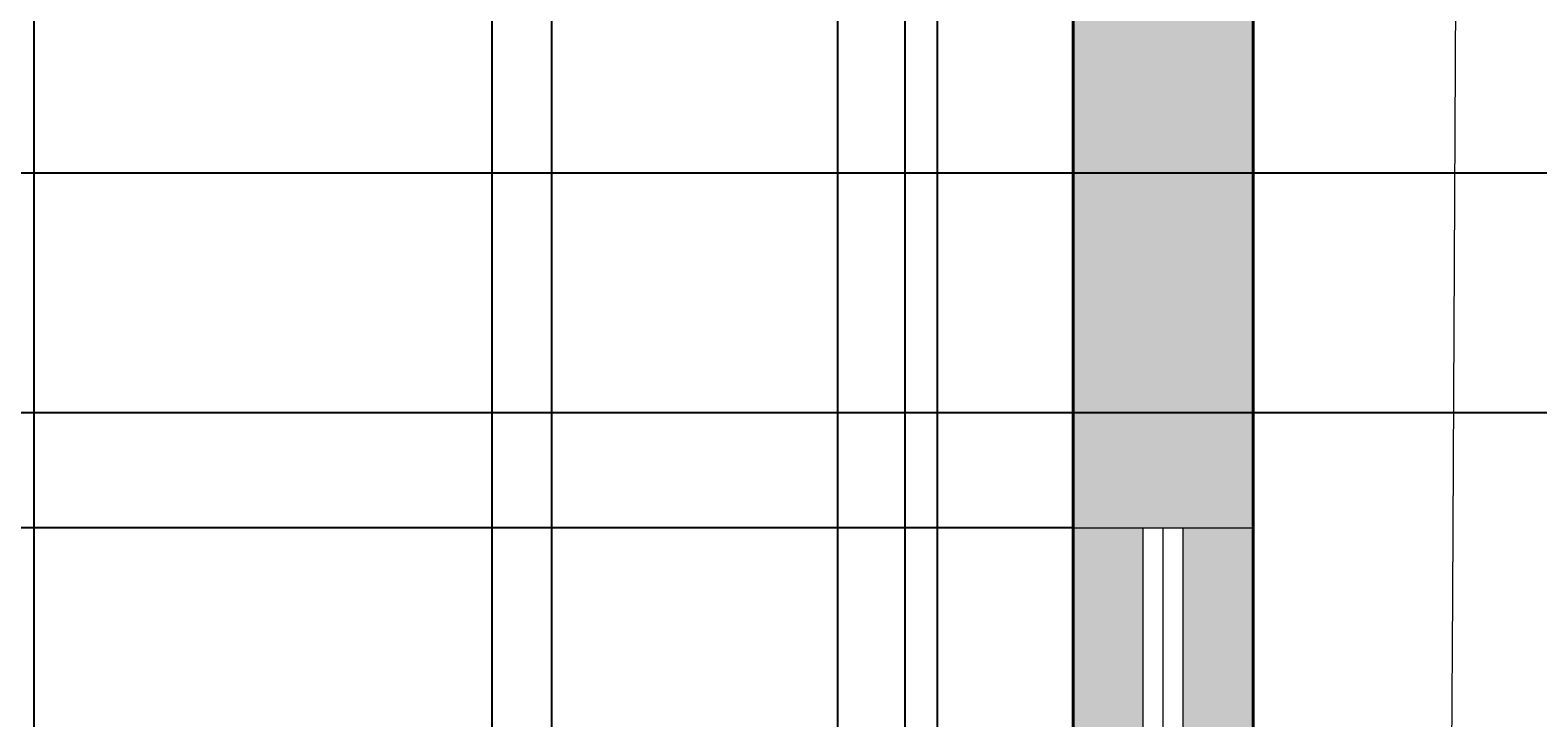
# Model space of a CAD drawing. Units: inches. Extents: x 818 to 1898, y 976 to 2364.
# Tile 30 of 96: x 1207 to 1282, y 1746 to 1780. Entities that reach past the tile are written whole.
import ezdxf

# ---------------------------------------------------------------- set-up
doc = ezdxf.new("R2010")
doc.units = ezdxf.units.IN
doc.header["$LTSCALE"] = 5
doc.header["$MEASUREMENT"] = 0
for name, color, linetype, lineweight in [('A-ANNO-DIMS', 2, 'Continuous', 18), ('A-FURN', 8, 'Continuous', 18), ('A-GLAZ', 4, 'Continuous', 18), ('A-WALL', 7, 'Continuous', 40)]:
    doc.layers.add(name, color=color, linetype=linetype, lineweight=lineweight)
doc.layers.add('A-GLAZ-PATT', color=141, linetype='Continuous', lineweight=9, true_color=0xadddf7)
doc.layers.add('A-WALL-PATT', color=251, linetype='Continuous', lineweight=13, true_color=0x636466)
doc.styles.get("Standard").update_dxf_attribs({"font": 'arial.ttf'})
doc.dimstyles.get("Standard").update_dxf_attribs({"dimtxt": 0.18, "dimasz": 0.18, "dimexe": 0.18, "dimexo": 0.0625, "dimgap": 0.09, "dimtad": 0, "dimtih": 1, "dimtoh": 1, "dimdec": 4, "dimzin": 0, "dimdsep": 46, "dimtxsty": 'Standard', "dimcen": 0.09, "dimadec": 0, "dimazin": 0, "dimtfac": 1, "dimtdec": 4, "dimtofl": 0, "dimtmove": 0, "dimatfit": 3, "dimfxl": 1, "dimtolj": 1, "dimtzin": 0, "dimarcsym": 0})

# ---------------------------------------------------------------- blocks, each defined once
blk = doc.blocks.new('SOFA-3-SEAT')
for p, q in [((39.87, 35.861), (5.697, 36.046)), ((74.051, 35.676), (39.879, 35.861))]:
    blk.add_line(p, q)
blk = doc.blocks.new('*D59')
at = {"layer": 'A-ANNO-DIMS', "color": 0, "lineweight": -2, "ltscale": 5, "transparency": 16777216}
for p, q in [((1251.643, 2300.393), (818.026, 2300.393)), ((818.206, 2300.213), (818.206, 1669.95)), ((818.206, 1039.323), (818.206, 1669.586)), ((896.051, 1039.143), (818.026, 1039.143))]:
    blk.add_line(p, q, dxfattribs=at)
at = {"layer": 'A-ANNO-DIMS', "color": 0, "ltscale": 5, "transparency": 16777216}
for points in [[(818.176, 2300.213), (818.236, 2300.213), (818.206, 2300.393)], [(818.176, 1039.323), (818.236, 1039.323), (818.206, 1039.143)]]:
    blk.add_solid(points, dxfattribs=at)
at = {"layer": 'Defpoints', "color": 0, "ltscale": 5, "transparency": 16777216}
for p in [(818.206, 2300.393), (1251.706, 2300.393), (896.114, 1039.143)]:
    blk.add_point(p, dxfattribs=at)
at = {"layer": 'A-ANNO-DIMS', "color": 0, "ltscale": 5, "transparency": 16777216, "insert": (818.206, 1669.768), "char_height": 0.18, "attachment_point": 5}
blk.add_mtext('\\A1;1261.2', dxfattribs=at)
blk = doc.blocks.new('*D61')
at = {"layer": 'A-ANNO-DIMS', "color": 0, "lineweight": -2, "ltscale": 5, "transparency": 16777216}
for p, q in [((1071.725, 1203.027), (1071.725, 2363.873)), ((1430.725, 1203.027), (1430.725, 2363.873)), ((1071.905, 2363.693), (1250.936, 2363.693)), ((1430.545, 2363.693), (1251.514, 2363.693))]:
    blk.add_line(p, q, dxfattribs=at)
at = {"layer": 'A-ANNO-DIMS', "color": 0, "ltscale": 5, "transparency": 16777216}
for points in [[(1071.905, 2363.723), (1071.905, 2363.663), (1071.725, 2363.693)], [(1430.545, 2363.723), (1430.545, 2363.663), (1430.725, 2363.693)]]:
    blk.add_solid(points, dxfattribs=at)
at = {"layer": 'Defpoints', "color": 0, "ltscale": 5, "transparency": 16777216}
for p in [(1430.725, 2363.693), (1071.725, 1202.964), (1430.725, 1202.964)]:
    blk.add_point(p, dxfattribs=at)
at = {"layer": 'A-ANNO-DIMS', "color": 0, "ltscale": 5, "transparency": 16777216, "insert": (1251.225, 2363.693), "char_height": 0.18, "attachment_point": 5}
blk.add_mtext('\\A1;359', dxfattribs=at)
blk = doc.blocks.new('*D64')
at = {"layer": 'A-ANNO-DIMS', "color": 0, "lineweight": -2, "ltscale": 5, "transparency": 16777216}
for p, q in [((1197.725, 1501.141), (1197.725, 2363.873)), ((1430.725, 1501.141), (1430.725, 2363.873)), ((1197.905, 2363.693), (1313.935, 2363.693)), ((1430.545, 2363.693), (1314.516, 2363.693))]:
    blk.add_line(p, q, dxfattribs=at)
at = {"layer": 'A-ANNO-DIMS', "color": 0, "ltscale": 5, "transparency": 16777216}
for points in [[(1197.905, 2363.723), (1197.905, 2363.663), (1197.725, 2363.693)], [(1430.545, 2363.723), (1430.545, 2363.663), (1430.725, 2363.693)]]:
    blk.add_solid(points, dxfattribs=at)
at = {"layer": 'Defpoints', "color": 0, "ltscale": 5, "transparency": 16777216}
for p in [(1430.725, 2363.693), (1197.725, 1501.078), (1430.725, 1501.078)]:
    blk.add_point(p, dxfattribs=at)
at = {"layer": 'A-ANNO-DIMS', "color": 0, "ltscale": 5, "transparency": 16777216, "insert": (1314.225, 2363.693), "char_height": 0.18, "attachment_point": 5}
blk.add_mtext('\\A1;233', dxfattribs=at)
blk = doc.blocks.new('*D83')
at = {"layer": 'A-ANNO-DIMS', "color": 0, "lineweight": -2, "ltscale": 5, "transparency": 16777216}
for p, q in [((1197.725, 1700.141), (1197.725, 2363.873)), ((1258.725, 1700.141), (1258.725, 2363.873)), ((1197.905, 2363.693), (1228.023, 2363.693)), ((1258.545, 2363.693), (1228.427, 2363.693))]:
    blk.add_line(p, q, dxfattribs=at)
at = {"layer": 'A-ANNO-DIMS', "color": 0, "ltscale": 5, "transparency": 16777216}
for points in [[(1197.905, 2363.723), (1197.905, 2363.663), (1197.725, 2363.693)], [(1258.545, 2363.723), (1258.545, 2363.663), (1258.725, 2363.693)]]:
    blk.add_solid(points, dxfattribs=at)
at = {"layer": 'Defpoints', "color": 0, "ltscale": 5, "transparency": 16777216}
for p in [(1258.725, 2363.693), (1197.725, 1700.078), (1258.725, 1700.078)]:
    blk.add_point(p, dxfattribs=at)
at = {"layer": 'A-ANNO-DIMS', "color": 0, "ltscale": 5, "transparency": 16777216, "insert": (1228.225, 2363.693), "char_height": 0.18, "attachment_point": 5}
blk.add_mtext('\\A1;61', dxfattribs=at)
blk = doc.blocks.new('*D85')
at = {"layer": 'A-ANNO-DIMS', "color": 0, "lineweight": -2, "ltscale": 5, "transparency": 16777216}
for p, q in [((1258.788, 2053.078), (1897.916, 2053.078)), ((1897.736, 2052.898), (1897.736, 1876.76)), ((1897.736, 1700.258), (1897.736, 1876.396)), ((1258.788, 1700.078), (1897.916, 1700.078))]:
    blk.add_line(p, q, dxfattribs=at)
at = {"layer": 'A-ANNO-DIMS', "color": 0, "ltscale": 5, "transparency": 16777216}
for points in [[(1897.706, 2052.898), (1897.766, 2052.898), (1897.736, 2053.078)], [(1897.706, 1700.258), (1897.766, 1700.258), (1897.736, 1700.078)]]:
    blk.add_solid(points, dxfattribs=at)
at = {"layer": 'Defpoints', "color": 0, "ltscale": 5, "transparency": 16777216}
for p in [(1258.725, 2053.078), (1897.736, 2053.078), (1258.725, 1700.078)]:
    blk.add_point(p, dxfattribs=at)
at = {"layer": 'A-ANNO-DIMS', "color": 0, "ltscale": 5, "transparency": 16777216, "insert": (1897.736, 1876.578), "char_height": 0.18, "attachment_point": 5}
blk.add_mtext('\\A1;353', dxfattribs=at)
blk = doc.blocks.new('*D95')
at = {"layer": 'A-ANNO-DIMS', "color": 0, "lineweight": -2, "ltscale": 5, "transparency": 16777216}
for p, q in [((1173.542, 1071.118), (1173.542, 2363.873)), ((1229.647, 1071.118), (1229.647, 2363.873)), ((1173.722, 2363.693), (1201.288, 2363.693)), ((1229.467, 2363.693), (1201.901, 2363.693))]:
    blk.add_line(p, q, dxfattribs=at)
at = {"layer": 'A-ANNO-DIMS', "color": 0, "ltscale": 5, "transparency": 16777216}
for points in [[(1173.722, 2363.723), (1173.722, 2363.663), (1173.542, 2363.693)], [(1229.467, 2363.723), (1229.467, 2363.663), (1229.647, 2363.693)]]:
    blk.add_solid(points, dxfattribs=at)
at = {"layer": 'Defpoints', "color": 0, "ltscale": 5, "transparency": 16777216}
for p in [(1229.647, 2363.693), (1173.542, 1071.055), (1229.647, 1071.055)]:
    blk.add_point(p, dxfattribs=at)
at = {"layer": 'A-ANNO-DIMS', "color": 0, "ltscale": 5, "transparency": 16777216, "insert": (1201.595, 2363.693), "char_height": 0.18, "attachment_point": 5}
blk.add_mtext('\\A1;56.1', dxfattribs=at)
blk = doc.blocks.new('*D96')
at = {"layer": 'A-ANNO-DIMS', "color": 0, "lineweight": -2, "ltscale": 5, "transparency": 16777216}
for p, q in [((1229.647, 1071.118), (1229.647, 2363.873)), ((1284.17, 1071.118), (1284.17, 2363.873)), ((1229.827, 2363.693), (1256.516, 2363.693)), ((1283.99, 2363.693), (1257.301, 2363.693))]:
    blk.add_line(p, q, dxfattribs=at)
at = {"layer": 'A-ANNO-DIMS', "color": 0, "ltscale": 5, "transparency": 16777216}
for points in [[(1229.827, 2363.723), (1229.827, 2363.663), (1229.647, 2363.693)], [(1283.99, 2363.723), (1283.99, 2363.663), (1284.17, 2363.693)]]:
    blk.add_solid(points, dxfattribs=at)
at = {"layer": 'Defpoints', "color": 0, "ltscale": 5, "transparency": 16777216}
for p in [(1284.17, 2363.693), (1229.647, 1071.055), (1284.17, 1071.055)]:
    blk.add_point(p, dxfattribs=at)
at = {"layer": 'A-ANNO-DIMS', "color": 0, "ltscale": 5, "transparency": 16777216, "insert": (1256.909, 2363.693), "char_height": 0.18, "attachment_point": 5}
blk.add_mtext('\\A1;54.52', dxfattribs=at)
blk = doc.blocks.new('*D120')
at = {"layer": 'A-ANNO-DIMS', "color": 0, "lineweight": -2, "ltscale": 5, "transparency": 16777216}
for p, q in [((1766.29, 1797.717), (818.026, 1797.717)), ((818.206, 1797.537), (818.206, 1757.534)), ((818.206, 1717.167), (818.206, 1757.17)), ((1766.29, 1716.987), (818.026, 1716.987))]:
    blk.add_line(p, q, dxfattribs=at)
at = {"layer": 'A-ANNO-DIMS', "color": 0, "ltscale": 5, "transparency": 16777216}
for points in [[(818.176, 1797.537), (818.236, 1797.537), (818.206, 1797.717)], [(818.176, 1717.167), (818.236, 1717.167), (818.206, 1716.987)]]:
    blk.add_solid(points, dxfattribs=at)
at = {"layer": 'Defpoints', "color": 0, "ltscale": 5, "transparency": 16777216}
for p in [(818.206, 1797.717), (1766.352, 1797.717), (1766.352, 1716.987)]:
    blk.add_point(p, dxfattribs=at)
at = {"layer": 'A-ANNO-DIMS', "color": 0, "ltscale": 5, "transparency": 16777216, "insert": (818.206, 1757.352), "char_height": 0.18, "attachment_point": 5}
blk.add_mtext('\\A1;80.73', dxfattribs=at)
blk = doc.blocks.new('*D145')
at = {"layer": 'A-ANNO-DIMS', "color": 0, "lineweight": -2, "ltscale": 5, "transparency": 16777216}
for p, q in [((1197.393, 2122.314), (1197.393, 975.663)), ((1232.609, 2122.314), (1232.609, 975.663)), ((1197.573, 975.843), (1214.608, 975.843)), ((1232.429, 975.843), (1215.394, 975.843))]:
    blk.add_line(p, q, dxfattribs=at)
at = {"layer": 'A-ANNO-DIMS', "color": 0, "ltscale": 5, "transparency": 16777216}
for points in [[(1197.573, 975.873), (1197.573, 975.813), (1197.393, 975.843)], [(1232.429, 975.873), (1232.429, 975.813), (1232.609, 975.843)]]:
    blk.add_solid(points, dxfattribs=at)
at = {"layer": 'Defpoints', "color": 0, "ltscale": 5, "transparency": 16777216}
for p in [(1197.393, 2122.377), (1232.609, 2122.377), (1232.609, 975.843)]:
    blk.add_point(p, dxfattribs=at)
at = {"layer": 'A-ANNO-DIMS', "color": 0, "ltscale": 5, "transparency": 16777216, "insert": (1215.001, 975.843), "char_height": 0.18, "attachment_point": 5}
blk.add_mtext('\\A1;35.22', dxfattribs=at)
blk = doc.blocks.new('*D215')
at = {"layer": 'A-ANNO-DIMS', "color": 0, "lineweight": -2, "ltscale": 5, "transparency": 16777216}
for p, q in [((1590.663, 1876.078), (818.026, 1876.078)), ((818.206, 1875.898), (818.206, 1781.76)), ((818.206, 1687.258), (818.206, 1781.396)), ((1511.663, 1687.078), (818.026, 1687.078))]:
    blk.add_line(p, q, dxfattribs=at)
at = {"layer": 'A-ANNO-DIMS', "color": 0, "ltscale": 5, "transparency": 16777216}
for points in [[(818.176, 1875.898), (818.236, 1875.898), (818.206, 1876.078)], [(818.176, 1687.258), (818.236, 1687.258), (818.206, 1687.078)]]:
    blk.add_solid(points, dxfattribs=at)
at = {"layer": 'Defpoints', "color": 0, "ltscale": 5, "transparency": 16777216}
for p in [(818.206, 1876.078), (1590.725, 1876.078), (1511.725, 1687.078)]:
    blk.add_point(p, dxfattribs=at)
at = {"layer": 'A-ANNO-DIMS', "color": 0, "ltscale": 5, "transparency": 16777216, "insert": (818.206, 1781.578), "char_height": 0.18, "attachment_point": 5}
blk.add_mtext('\\A1;189', dxfattribs=at)
blk = doc.blocks.new('*D220')
at = {"layer": 'A-ANNO-DIMS', "color": 0, "lineweight": -2, "ltscale": 5, "transparency": 16777216}
for p, q in [((1520.663, 1773.078), (818.026, 1773.078)), ((818.206, 1772.898), (818.206, 1767.259)), ((818.206, 1761.258), (818.206, 1766.898)), ((1520.663, 1761.078), (818.026, 1761.078))]:
    blk.add_line(p, q, dxfattribs=at)
at = {"layer": 'A-ANNO-DIMS', "color": 0, "ltscale": 5, "transparency": 16777216}
for points in [[(818.176, 1772.898), (818.236, 1772.898), (818.206, 1773.078)], [(818.176, 1761.258), (818.236, 1761.258), (818.206, 1761.078)]]:
    blk.add_solid(points, dxfattribs=at)
at = {"layer": 'Defpoints', "color": 0, "ltscale": 5, "transparency": 16777216}
for p in [(818.206, 1773.078), (1520.725, 1773.078), (1520.725, 1761.078)]:
    blk.add_point(p, dxfattribs=at)
at = {"layer": 'A-ANNO-DIMS', "color": 0, "ltscale": 5, "transparency": 16777216, "insert": (818.206, 1767.078), "char_height": 0.18, "attachment_point": 5}
blk.add_mtext('\\A1;12', dxfattribs=at)
blk = doc.blocks.new('*D233')
at = {"layer": 'A-ANNO-DIMS', "color": 0, "lineweight": -2, "ltscale": 5, "transparency": 16777216}
for p, q in [((1267.725, 2044.016), (1267.725, 975.663)), ((1303.931, 2008.329), (1303.931, 975.663)), ((1267.905, 975.843), (1285.365, 975.843)), ((1303.751, 975.843), (1286.292, 975.843))]:
    blk.add_line(p, q, dxfattribs=at)
at = {"layer": 'A-ANNO-DIMS', "color": 0, "ltscale": 5, "transparency": 16777216}
for points in [[(1267.905, 975.873), (1267.905, 975.813), (1267.725, 975.843)], [(1303.751, 975.873), (1303.751, 975.813), (1303.931, 975.843)]]:
    blk.add_solid(points, dxfattribs=at)
at = {"layer": 'Defpoints', "color": 0, "ltscale": 5, "transparency": 16777216}
for p in [(1267.725, 2044.078), (1303.931, 2008.392), (1303.931, 975.843)]:
    blk.add_point(p, dxfattribs=at)
at = {"layer": 'A-ANNO-DIMS', "color": 0, "ltscale": 5, "transparency": 16777216, "insert": (1285.828, 975.843), "char_height": 0.18, "attachment_point": 5}
blk.add_mtext('\\A1;36.206', dxfattribs=at)
blk = doc.blocks.new('*D246')
at = {"layer": 'A-ANNO-DIMS', "color": 0, "lineweight": -2, "ltscale": 5, "transparency": 16777216}
for p, q in [((1258.663, 1755.332), (818.026, 1755.332)), ((818.206, 1755.152), (818.206, 1731.514)), ((818.206, 1707.512), (818.206, 1731.15)), ((1258.663, 1707.332), (818.026, 1707.332))]:
    blk.add_line(p, q, dxfattribs=at)
at = {"layer": 'A-ANNO-DIMS', "color": 0, "ltscale": 5, "transparency": 16777216}
for points in [[(818.176, 1755.152), (818.236, 1755.152), (818.206, 1755.332)], [(818.176, 1707.512), (818.236, 1707.512), (818.206, 1707.332)]]:
    blk.add_solid(points, dxfattribs=at)
at = {"layer": 'Defpoints', "color": 0, "ltscale": 5, "transparency": 16777216}
for p in [(818.206, 1755.332), (1258.725, 1755.332), (1258.725, 1707.332)]:
    blk.add_point(p, dxfattribs=at)
at = {"layer": 'A-ANNO-DIMS', "color": 0, "ltscale": 5, "transparency": 16777216, "insert": (818.206, 1731.332), "char_height": 0.18, "attachment_point": 5}
blk.add_mtext('\\A1;48', dxfattribs=at)
blk = doc.blocks.new('*D249')
at = {"layer": 'A-ANNO-DIMS', "color": 0, "lineweight": -2, "ltscale": 5, "transparency": 16777216}
for p, q in [((1258.663, 1814.965), (818.026, 1814.965)), ((818.206, 1814.785), (818.206, 1785.331)), ((818.206, 1755.512), (818.206, 1784.967)), ((1258.663, 1755.332), (818.026, 1755.332))]:
    blk.add_line(p, q, dxfattribs=at)
at = {"layer": 'A-ANNO-DIMS', "color": 0, "ltscale": 5, "transparency": 16777216}
for points in [[(818.176, 1814.785), (818.236, 1814.785), (818.206, 1814.965)], [(818.176, 1755.512), (818.236, 1755.512), (818.206, 1755.332)]]:
    blk.add_solid(points, dxfattribs=at)
at = {"layer": 'Defpoints', "color": 0, "ltscale": 5, "transparency": 16777216}
for p in [(818.206, 1814.965), (1258.725, 1814.965), (1258.725, 1755.332)]:
    blk.add_point(p, dxfattribs=at)
at = {"layer": 'A-ANNO-DIMS', "color": 0, "ltscale": 5, "transparency": 16777216, "insert": (818.206, 1785.149), "char_height": 0.18, "attachment_point": 5}
blk.add_mtext('\\A1;59.63', dxfattribs=at)
blk = doc.blocks.new('*D251')
at = {"layer": 'A-ANNO-DIMS', "color": 0, "lineweight": -2, "ltscale": 5, "transparency": 16777216}
for p, q in [((1250.303, 1878.329), (1250.303, 975.663)), ((1258.725, 1878.329), (1258.725, 975.663)), ((1250.483, 975.843), (1254.121, 975.843)), ((1258.545, 975.843), (1254.907, 975.843))]:
    blk.add_line(p, q, dxfattribs=at)
at = {"layer": 'A-ANNO-DIMS', "color": 0, "ltscale": 5, "transparency": 16777216}
for points in [[(1250.483, 975.873), (1250.483, 975.813), (1250.303, 975.843)], [(1258.545, 975.873), (1258.545, 975.813), (1258.725, 975.843)]]:
    blk.add_solid(points, dxfattribs=at)
at = {"layer": 'Defpoints', "color": 0, "ltscale": 5, "transparency": 16777216}
for p in [(1250.303, 1878.392), (1258.725, 1878.392), (1258.725, 975.843)]:
    blk.add_point(p, dxfattribs=at)
at = {"layer": 'A-ANNO-DIMS', "color": 0, "ltscale": 5, "transparency": 16777216, "insert": (1254.514, 975.843), "char_height": 0.18, "attachment_point": 5}
blk.add_mtext('\\A1;8.422', dxfattribs=at)
blk = doc.blocks.new('*D254')
at = {"layer": 'A-ANNO-DIMS', "color": 0, "lineweight": -2, "ltscale": 5, "transparency": 16777216}
for p, q in [((1267.725, 2044.016), (1267.725, 975.663)), ((1330.305, 2044.016), (1330.305, 975.663)), ((1267.905, 975.843), (1298.621, 975.843)), ((1330.125, 975.843), (1299.409, 975.843))]:
    blk.add_line(p, q, dxfattribs=at)
at = {"layer": 'A-ANNO-DIMS', "color": 0, "ltscale": 5, "transparency": 16777216}
for points in [[(1267.905, 975.873), (1267.905, 975.813), (1267.725, 975.843)], [(1330.125, 975.873), (1330.125, 975.813), (1330.305, 975.843)]]:
    blk.add_solid(points, dxfattribs=at)
at = {"layer": 'Defpoints', "color": 0, "ltscale": 5, "transparency": 16777216}
for p in [(1267.725, 2044.078), (1330.305, 2044.078), (1330.305, 975.843)]:
    blk.add_point(p, dxfattribs=at)
at = {"layer": 'A-ANNO-DIMS', "color": 0, "ltscale": 5, "transparency": 16777216, "insert": (1299.015, 975.843), "char_height": 0.18, "attachment_point": 5}
blk.add_mtext('\\A1;62.58', dxfattribs=at)
blk = doc.blocks.new('*D269')
at = {"layer": 'A-ANNO-DIMS', "color": 0, "lineweight": -2, "ltscale": 5, "transparency": 16777216}
for p, q in [((1246.938, 1534.141), (1246.938, 2363.873)), ((1341.259, 1534.141), (1341.259, 2363.873)), ((1247.118, 2363.693), (1293.706, 2363.693)), ((1341.079, 2363.693), (1294.491, 2363.693))]:
    blk.add_line(p, q, dxfattribs=at)
at = {"layer": 'A-ANNO-DIMS', "color": 0, "ltscale": 5, "transparency": 16777216}
for points in [[(1247.118, 2363.723), (1247.118, 2363.663), (1246.938, 2363.693)], [(1341.079, 2363.723), (1341.079, 2363.663), (1341.259, 2363.693)]]:
    blk.add_solid(points, dxfattribs=at)
at = {"layer": 'Defpoints', "color": 0, "ltscale": 5, "transparency": 16777216}
for p in [(1341.259, 2363.693), (1246.938, 1534.078), (1341.259, 1534.078)]:
    blk.add_point(p, dxfattribs=at)
at = {"layer": 'A-ANNO-DIMS', "color": 0, "ltscale": 5, "transparency": 16777216, "insert": (1294.099, 2363.693), "char_height": 0.18, "attachment_point": 5}
blk.add_mtext('\\A1;94.32', dxfattribs=at)
blk = doc.blocks.new('*D271')
at = {"layer": 'A-ANNO-DIMS', "color": 0, "lineweight": -2, "ltscale": 5, "transparency": 16777216}
for p, q in [((1206.725, 1510.141), (1206.725, 2363.873)), ((1246.938, 1510.141), (1246.938, 2363.873)), ((1206.905, 2363.693), (1226.451, 2363.693)), ((1246.758, 2363.693), (1227.211, 2363.693))]:
    blk.add_line(p, q, dxfattribs=at)
at = {"layer": 'A-ANNO-DIMS', "color": 0, "ltscale": 5, "transparency": 16777216}
for points in [[(1206.905, 2363.723), (1206.905, 2363.663), (1206.725, 2363.693)], [(1246.758, 2363.723), (1246.758, 2363.663), (1246.938, 2363.693)]]:
    blk.add_solid(points, dxfattribs=at)
at = {"layer": 'Defpoints', "color": 0, "ltscale": 5, "transparency": 16777216}
for p in [(1246.938, 2363.693), (1206.725, 1510.078), (1246.938, 1510.078)]:
    blk.add_point(p, dxfattribs=at)
at = {"layer": 'A-ANNO-DIMS', "color": 0, "ltscale": 5, "transparency": 16777216, "insert": (1226.831, 2363.693), "char_height": 0.18, "attachment_point": 5}
blk.add_mtext('\\A1;40.21', dxfattribs=at)
blk = doc.blocks.new('*D276')
at = {"layer": 'A-ANNO-DIMS', "color": 0, "lineweight": -2, "ltscale": 5, "transparency": 16777216}
for p, q in [((1206.725, 1687.141), (1206.725, 2363.873)), ((1251.933, 1681.439), (1251.933, 2363.873)), ((1206.905, 2363.693), (1228.949, 2363.693)), ((1251.753, 2363.693), (1229.709, 2363.693))]:
    blk.add_line(p, q, dxfattribs=at)
at = {"layer": 'A-ANNO-DIMS', "color": 0, "ltscale": 5, "transparency": 16777216}
for points in [[(1206.905, 2363.723), (1206.905, 2363.663), (1206.725, 2363.693)], [(1251.753, 2363.723), (1251.753, 2363.663), (1251.933, 2363.693)]]:
    blk.add_solid(points, dxfattribs=at)
at = {"layer": 'Defpoints', "color": 0, "ltscale": 5, "transparency": 16777216}
for p in [(1251.933, 2363.693), (1206.725, 1687.078), (1251.933, 1681.376)]:
    blk.add_point(p, dxfattribs=at)
at = {"layer": 'A-ANNO-DIMS', "color": 0, "ltscale": 5, "transparency": 16777216, "insert": (1229.329, 2363.693), "char_height": 0.18, "attachment_point": 5}
blk.add_mtext('\\A1;45.21', dxfattribs=at)
blk = doc.blocks.new('*D283')
at = {"layer": 'A-ANNO-DIMS', "color": 0, "lineweight": -2, "ltscale": 5, "transparency": 16777216}
for p, q in [((1351.599, 1761.386), (1351.599, 975.663)), ((1267.725, 1696.016), (1267.725, 975.663)), ((1267.905, 975.843), (1309.268, 975.843)), ((1351.419, 975.843), (1310.056, 975.843))]:
    blk.add_line(p, q, dxfattribs=at)
at = {"layer": 'A-ANNO-DIMS', "color": 0, "ltscale": 5, "transparency": 16777216}
for points in [[(1267.905, 975.873), (1267.905, 975.813), (1267.725, 975.843)], [(1351.419, 975.873), (1351.419, 975.813), (1351.599, 975.843)]]:
    blk.add_solid(points, dxfattribs=at)
at = {"layer": 'Defpoints', "color": 0, "ltscale": 5, "transparency": 16777216}
for p in [(1351.599, 1761.449), (1267.725, 1696.078), (1351.599, 975.843)]:
    blk.add_point(p, dxfattribs=at)
at = {"layer": 'A-ANNO-DIMS', "color": 0, "ltscale": 5, "transparency": 16777216, "insert": (1309.662, 975.843), "char_height": 0.18, "attachment_point": 5}
blk.add_mtext('\\A1;83.87', dxfattribs=at)
blk = doc.blocks.new('*D284')
at = {"layer": 'A-ANNO-DIMS', "color": 0, "lineweight": -2, "ltscale": 5, "transparency": 16777216}
for p, q in [((1351.661, 1761.449), (1897.916, 1761.449)), ((1897.736, 1761.269), (1897.736, 1728.946)), ((1897.736, 1696.258), (1897.736, 1728.582)), ((1267.788, 1696.078), (1897.916, 1696.078))]:
    blk.add_line(p, q, dxfattribs=at)
at = {"layer": 'A-ANNO-DIMS', "color": 0, "ltscale": 5, "transparency": 16777216}
for points in [[(1897.706, 1761.269), (1897.766, 1761.269), (1897.736, 1761.449)], [(1897.706, 1696.258), (1897.766, 1696.258), (1897.736, 1696.078)]]:
    blk.add_solid(points, dxfattribs=at)
at = {"layer": 'Defpoints', "color": 0, "ltscale": 5, "transparency": 16777216}
for p in [(1351.599, 1761.449), (1267.725, 1696.078), (1897.736, 1696.078)]:
    blk.add_point(p, dxfattribs=at)
at = {"layer": 'A-ANNO-DIMS', "color": 0, "ltscale": 5, "transparency": 16777216, "insert": (1897.736, 1728.764), "char_height": 0.18, "attachment_point": 5}
blk.add_mtext('\\A1;65.37', dxfattribs=at)
blk = doc.blocks.new('*D285')
at = {"layer": 'A-ANNO-DIMS', "color": 0, "lineweight": -2, "ltscale": 5, "transparency": 16777216}
for p, q in [((1305.828, 1830.022), (1305.828, 975.663)), ((1267.725, 1814.903), (1267.725, 975.663)), ((1267.905, 975.843), (1286.47, 975.843)), ((1305.648, 975.843), (1287.083, 975.843))]:
    blk.add_line(p, q, dxfattribs=at)
at = {"layer": 'A-ANNO-DIMS', "color": 0, "ltscale": 5, "transparency": 16777216}
for points in [[(1267.905, 975.873), (1267.905, 975.813), (1267.725, 975.843)], [(1305.648, 975.873), (1305.648, 975.813), (1305.828, 975.843)]]:
    blk.add_solid(points, dxfattribs=at)
at = {"layer": 'Defpoints', "color": 0, "ltscale": 5, "transparency": 16777216}
for p in [(1305.828, 1830.084), (1267.725, 1814.965), (1267.725, 975.843)]:
    blk.add_point(p, dxfattribs=at)
at = {"layer": 'A-ANNO-DIMS', "color": 0, "ltscale": 5, "transparency": 16777216, "insert": (1286.776, 975.843), "char_height": 0.18, "attachment_point": 5}
blk.add_mtext('\\A1;38.1', dxfattribs=at)

msp = doc.modelspace()

# ---------------------------------------------------------------- hatches: boundary and pattern name
at = {"layer": 'A-GLAZ-PATT', "ltscale": 5}
h = msp.add_hatch(color=256, dxfattribs=at)
h.dxf.hatch_style = 1
h.paths.add_polyline_path([(1283.8183, 1504.5782), (1206.7251, 1504.5782), (1206.7251, 1501.0782), (1283.8183, 1501.0782)])
h.paths.add_polyline_path([(1283.8183, 1510.0782), (1206.7251, 1510.0782), (1206.7251, 1506.5782), (1283.8183, 1506.5782)])
h.paths.add_polyline_path([(1490.9163, 1355.0782), (1439.7252, 1355.0782), (1439.7252, 1409.0522), (1436.2252, 1409.0522), (1436.2252, 1351.5782), (1490.9163, 1351.5782)])
h.paths.add_polyline_path([(1434.2252, 1409.0522), (1430.7251, 1409.0522), (1430.7251, 1346.0782), (1435.0799, 1346.0782), (1435.0731, 1346.1152), (1435.1501, 1346.0782), (1490.9163, 1346.0782), (1490.9163, 1349.5782), (1434.2252, 1349.5782)])
h.paths.add_polyline_path([(1714.7252, 1545.0782), (1711.2252, 1545.0782), (1711.2252, 1521.0782), (1714.7252, 1521.0782)])
h.paths.add_polyline_path([(1709.2252, 1545.0782), (1705.7252, 1545.0782), (1705.7252, 1521.0782), (1709.2252, 1521.0782)])
h.paths.add_polyline_path([(1714.7252, 1687.0782), (1711.2252, 1687.0782), (1711.2252, 1649.9029), (1714.7252, 1649.9029)])
h.paths.add_polyline_path([(1709.2252, 1687.0782), (1705.7252, 1687.0782), (1705.7252, 1649.9029), (1709.2252, 1649.9029)])
h.paths.add_polyline_path([(1709.2252, 1745.5584), (1705.7252, 1745.5584), (1705.7252, 1717.3178), (1709.2252, 1717.3178)])
h.paths.add_polyline_path([(1714.7252, 1745.5584), (1711.2252, 1745.5584), (1711.2252, 1717.3178), (1714.7252, 1717.3178)])
h.paths.add_polyline_path([(1714.7252, 2014.5114), (1711.2252, 2014.5114), (1711.2252, 1962.0338), (1714.7252, 1962.0338)])
h.paths.add_polyline_path([(1709.2252, 2014.5114), (1705.7252, 2014.5114), (1705.7252, 1962.0338), (1709.2252, 1962.0338)])
h.paths.add_polyline_path([(1538.5155, 2047.5782), (1485.1216, 2047.5782), (1485.1216, 2044.0782), (1538.5155, 2044.0782)])
h.paths.add_polyline_path([(1538.5155, 2053.0782), (1485.1216, 2053.0782), (1485.1216, 2049.5782), (1538.5155, 2049.5782)])
h.paths.add_polyline_path([(1388.0315, 2047.5782), (1330.305, 2047.5782), (1330.305, 2044.0782), (1388.0315, 2044.0782)])
h.paths.add_polyline_path([(1388.0315, 2053.0782), (1330.305, 2053.0782), (1330.305, 2049.5782), (1388.0315, 2049.5782)])
h.paths.add_polyline_path([(1262.2252, 2019.2871), (1258.7251, 2019.2871), (1258.7251, 1928.9218), (1262.2252, 1928.9218)])
h.paths.add_polyline_path([(1267.7251, 2019.2871), (1264.2252, 2019.2871), (1264.2252, 1928.9218), (1267.7251, 1928.9218)])
h.paths.add_polyline_path([(1262.2252, 1862.9652), (1258.7251, 1862.9652), (1258.7251, 1814.9652), (1262.2252, 1814.9652)])
h.paths.add_polyline_path([(1267.7251, 1862.9652), (1264.2252, 1862.9652), (1264.2252, 1814.9652), (1267.7251, 1814.9652)])
h.paths.add_polyline_path([(1262.2252, 1755.3321), (1258.7251, 1755.3321), (1258.7251, 1707.3321), (1262.2252, 1707.3321)])
h.paths.add_polyline_path([(1267.7251, 1755.3321), (1264.2252, 1755.3321), (1264.2252, 1707.3321), (1267.7251, 1707.3321)])
h.paths.add_polyline_path([(1251.9333, 1692.5782), (1206.7251, 1692.5782), (1206.7251, 1687.0782), (1251.9333, 1687.0782)])
h.paths.add_polyline_path([(1251.9333, 1700.0782), (1206.7251, 1700.0782), (1206.7251, 1694.5782), (1251.9333, 1694.5782)])
at = {"layer": 'A-WALL-PATT', "ltscale": 5}
h = msp.add_hatch(color=256, dxfattribs=at)
h.dxf.hatch_style = 1
h.paths.add_polyline_path([(1267.7251, 1928.9218), (1258.7251, 1928.9218), (1258.7251, 1913.6401), (1250.3029, 1913.6401), (1250.3029, 1878.3919), (1258.7251, 1878.3919), (1258.7251, 1862.9652), (1267.7251, 1862.9652)])
h.paths.add_polyline_path([(1267.7251, 1814.9652), (1258.7251, 1814.9652), (1258.7251, 1755.3321), (1267.7251, 1755.3321)])
h.paths.add_polyline_path([(1463.7252, 1696.0782), (1267.7251, 1696.0782), (1267.7251, 1707.3321), (1258.7251, 1707.3321), (1258.7251, 1700.0782), (1251.9333, 1700.0782), (1251.9333, 1687.0782), (1463.7252, 1687.0782)])
h.paths.add_polyline_path([(1714.7252, 1717.3178), (1705.7252, 1717.3178), (1705.7252, 1696.0782), (1599.7252, 1696.0782), (1599.7252, 1790.0782), (1705.7252, 1790.0782), (1705.7252, 1785.6125), (1714.7252, 1785.6125), (1714.7252, 1827.2125), (1705.7252, 1827.2125), (1705.7252, 1802.0782), (1599.7252, 1802.0782), (1599.7252, 1867.0782), (1705.7252, 1867.0782), (1705.7252, 1857.2125), (1714.7252, 1857.2125), (1714.7252, 1930.0316), (1741.8409, 1930.0316), (1741.8409, 1935.0316), (1714.7252, 1935.0316), (1714.7252, 1957.0338), (1741.8409, 1957.0338), (1741.8409, 1962.0338), (1714.7252, 1962.0338), (1705.7252, 1962.0338), (1705.7252, 1948.0782), (1599.7252, 1948.0782), (1599.7252, 1981.0782), (1590.7251, 1981.0782), (1590.7251, 1941.0782), (1620.7252, 1941.0782), (1705.7252, 1941.0782), (1705.7252, 1876.0782), (1599.7252, 1876.0782), (1599.7252, 1911.0782), (1590.7251, 1911.0782), (1590.7251, 1876.0782), (1429.2252, 1876.0782), (1429.2252, 1867.0782), (1511.7251, 1867.0782), (1528.593, 1867.0782), (1595.7252, 1867.0782), (1595.7252, 1773.0782), (1520.7251, 1773.0782), (1520.7251, 1837.5823), (1532.593, 1837.5823), (1532.593, 1867.0782), (1528.593, 1867.0782), (1528.593, 1841.5823), (1511.7251, 1841.5823), (1511.7251, 1744.9714), (1520.7251, 1744.9714), (1520.7251, 1761.0782), (1595.7252, 1761.0782), (1595.7252, 1696.0782), (1520.7251, 1696.0782), (1520.7251, 1716.0454), (1511.7251, 1716.0454), (1511.7251, 1696.0782), (1511.7251, 1687.0782), (1714.7252, 1687.0782)])
h.paths.add_polyline_path([(1714.7252, 2053.0782), (1714.7252, 2081.1881), (1709.7252, 2081.1881), (1709.7252, 2053.0782), (1681.6446, 2053.0782), (1681.6446, 2081.1881), (1676.6446, 2081.1881), (1676.6446, 2053.0782), (1538.5155, 2053.0782), (1538.5155, 2044.0782), (1590.7251, 2044.0782), (1590.7251, 2011.0782), (1599.7252, 2011.0782), (1599.7252, 2044.0782), (1705.7252, 2044.0782), (1705.7252, 2014.5114), (1714.7252, 2014.5114)])
h.paths.add_polyline_path([(1485.1216, 2053.0782), (1422.02, 2053.0782), (1422.02, 2081.1881), (1413.02, 2081.1881), (1413.02, 2053.0782), (1399.6356, 2053.0782), (1399.6356, 2081.1881), (1390.6356, 2081.1881), (1390.6356, 2053.0782), (1388.0315, 2053.0782), (1388.0315, 2044.0782), (1416.2743, 2044.0782), (1485.1216, 2044.0782)])
h.paths.add_polyline_path([(1330.305, 2053.0782), (1258.7251, 2053.0782), (1258.7251, 2019.2871), (1267.7251, 2019.2871), (1267.7251, 2044.0782), (1330.305, 2044.0782)])
h.paths.add_polyline_path([(1258.7251, 2053.0782), (1214.6577, 2053.0782), (1214.6577, 2044.0782), (1258.7251, 2044.0782)])
h.paths.add_polyline_path([(1214.6577, 2053.0782), (1180.349, 2053.0782), (1180.349, 2044.0782), (1214.6577, 2044.0782)])
h.paths.add_polyline_path([(1714.7252, 1639.5782), (1741.8409, 1639.5782), (1741.8409, 1643.5782), (1714.7252, 1643.5782), (1714.7252, 1649.9029), (1705.7252, 1649.9029), (1705.7252, 1600.0782), (1477.7252, 1600.0782), (1477.7252, 1591.0782), (1520.7251, 1591.0782), (1616.7252, 1591.0782), (1616.7252, 1416.6857), (1622.7252, 1416.6857), (1622.7252, 1463.0782), (1624.7252, 1463.0782), (1624.7252, 1467.0782), (1622.7252, 1467.0782), (1622.7252, 1591.0782), (1705.7252, 1591.0782), (1705.7252, 1545.0782), (1714.7252, 1545.0782), (1741.8409, 1545.0782), (1741.8409, 1549.0782), (1714.7252, 1549.0782), (1714.7252, 1593.9175), (1737.8409, 1593.9175), (1737.8409, 1597.9175), (1714.7252, 1597.9175)])
h.paths.add_polyline_path([(1674.9024, 2060.7419), (1714.7045, 2060.7419), (1714.7045, 2073.1061), (1674.9024, 2073.1061)], flags=25)
h.paths.add_polyline_path([(1394.5468, 2061.6618), (1422.2344, 2061.6618), (1422.2344, 2074.0261), (1394.5468, 2074.0261)], flags=24)

# ---------------------------------------------------------------- linework, layer by layer
at = {"layer": 'A-GLAZ'}
for p, q in [((1258.7251, 1755.3321), (1267.7251, 1755.3321)), ((1262.2252, 1707.3321), (1262.2252, 1755.3321)), ((1263.2252, 1707.3321), (1263.2252, 1755.3321)), ((1264.2252, 1707.3321), (1264.2252, 1755.3321))]:
    msp.add_line(p, q, dxfattribs=at)
at = {"layer": 'A-WALL'}
for p, q in [((1258.7251, 1878.3919), (1258.7251, 1700.0782)), ((1267.7251, 1867.0782), (1267.7251, 1696.0782))]:
    msp.add_line(p, q, dxfattribs=at)

# ---------------------------------------------------------------- block references
at = {"layer": 'A-FURN', "rotation": 90.0000000000007}
msp.add_blockref('SOFA-3-SEAT', (1313.5566, 1712.0791), dxfattribs=at)

# ---------------------------------------------------------------- dimensions: what is measured, and where the dimension line sits
at = {"layer": 'A-ANNO-DIMS', "ltscale": 5}
for base, p1, p2, override, picture, middle in [((1430.7251, 2363.6929), (1071.7251, 1202.9642), (1430.7251, 1202.9642), {"dimdec": 0, "dimlfac": 1, "dimrnd": 0, "dimzin": 0, "dimdsep": 46, "dimlunit": 2}, '*D61', (1251.2251, 2363.6929)), ((1229.6474, 2363.6929), (1173.5418, 1071.0552), (1229.6474, 1071.0552), {"dimdec": 1, "dimlfac": 1, "dimrnd": 0, "dimzin": 0, "dimdsep": 46, "dimlunit": 2}, '*D95', (1201.5946, 2363.6929)), ((1430.7251, 2363.6929), (1197.7251, 1501.0782), (1430.7251, 1501.0782), {"dimdec": 0, "dimlfac": 1, "dimrnd": 0, "dimzin": 0, "dimdsep": 46, "dimlunit": 2}, '*D64', (1314.2251, 2363.6929)), ((1258.7251, 2363.6929), (1197.7251, 1700.0782), (1258.7251, 1700.0782), {"dimdec": 0, "dimlfac": 1, "dimrnd": 0, "dimzin": 0, "dimdsep": 46, "dimlunit": 2}, '*D83', (1228.2251, 2363.6929)), ((1246.9377, 2363.6929), (1206.7251, 1510.0782), (1246.9377, 1510.0782), {"dimdec": 2, "dimlfac": 1, "dimrnd": 0, "dimzin": 0, "dimdsep": 46, "dimlunit": 2}, '*D271', (1226.8314, 2363.6929)), ((1251.9333, 2363.6929), (1206.7251, 1687.0782), (1251.9333, 1681.3763), {"dimdec": 2, "dimlfac": 1, "dimrnd": 0, "dimzin": 0, "dimdsep": 46, "dimlunit": 2}, '*D276', (1229.3292, 2363.6929)), ((1284.1697, 2363.6929), (1229.6474, 1071.0552), (1284.1697, 1071.0552), {"dimdec": 2, "dimlfac": 1, "dimrnd": 0, "dimzin": 0, "dimdsep": 46, "dimlunit": 2}, '*D96', (1256.9085, 2363.6929)), ((1341.2593, 2363.6929), (1246.9377, 1534.0782), (1341.2593, 1534.0782), {"dimdec": 2, "dimlfac": 1, "dimrnd": 0, "dimzin": 0, "dimdsep": 46, "dimlunit": 2}, '*D269', (1294.0985, 2363.6929)), ((1232.6091, 975.8433), (1197.3925, 2122.3767), (1232.6091, 2122.3767), {"dimdec": 2, "dimlfac": 1, "dimrnd": 0, "dimzin": 0, "dimdsep": 46, "dimlunit": 2}, '*D145', (1215.0008, 975.8433)), ((1303.9314, 975.8433), (1267.7251, 2044.0782), (1303.9314, 2008.3917), {"dimdec": 3, "dimlfac": 1, "dimrnd": 0, "dimzin": 0, "dimdsep": 46, "dimlunit": 2}, '*D233', (1285.8283, 975.8433)), ((1330.305, 975.8433), (1267.7251, 2044.0782), (1330.305, 2044.0782), {"dimdec": 2, "dimlfac": 1, "dimrnd": 0, "dimzin": 0, "dimdsep": 46, "dimlunit": 2}, '*D254', (1299.0151, 975.8433)), ((1258.7251, 975.8433), (1250.3029, 1878.3919), (1258.7251, 1878.3919), {"dimdec": 3, "dimlfac": 1, "dimrnd": 0, "dimzin": 0, "dimdsep": 46, "dimlunit": 2}, '*D251', (1254.514, 975.8433)), ((1267.7251, 975.8433), (1305.8278, 1830.0844), (1267.7251, 1814.9652), {"dimdec": 1, "dimlfac": 1, "dimrnd": 0, "dimzin": 0, "dimdsep": 46, "dimlunit": 2}, '*D285', (1286.7765, 975.8433)), ((1351.5985, 975.8433), (1267.7251, 1696.0782), (1351.5985, 1761.449), {"dimdec": 2, "dimlfac": 1, "dimrnd": 0, "dimzin": 0, "dimdsep": 46, "dimlunit": 2}, '*D283', (1309.6618, 975.8433))]:
    dim = msp.add_linear_dim(base=base, p1=p1, p2=p2, dimstyle='Standard', override=override, dxfattribs=at)
    dim.commit()
    dim.dimension.update_dxf_attribs({"geometry": picture, "text_midpoint": middle})
for base, p1, p2, override, picture, middle in [((818.2059, 2300.3929), (896.1138, 1039.1433), (1251.7057, 2300.3929), {"dimdec": 1, "dimlfac": 1, "dimrnd": 0, "dimzin": 0, "dimdsep": 46, "dimlunit": 2}, '*D59', (818.2059, 1669.7681)), ((1897.736, 2053.0782), (1258.7251, 1700.0782), (1258.7251, 2053.0782), {"dimdec": 0, "dimlfac": 1, "dimrnd": 0, "dimzin": 0, "dimdsep": 46, "dimlunit": 2}, '*D85', (1897.736, 1876.5782)), ((818.2059, 1876.0782), (1511.7251, 1687.0782), (1590.7251, 1876.0782), {"dimdec": 0, "dimlfac": 1, "dimrnd": 0, "dimzin": 0, "dimdsep": 46, "dimlunit": 2}, '*D215', (818.2059, 1781.5782)), ((818.2059, 1814.9652), (1258.7251, 1755.3321), (1258.7251, 1814.9652), {"dimdec": 2, "dimlfac": 1, "dimrnd": 0, "dimzin": 0, "dimdsep": 46, "dimlunit": 2}, '*D249', (818.2059, 1785.1486)), ((818.2059, 1797.7165), (1766.3524, 1716.9866), (1766.3524, 1797.7165), {"dimdec": 2, "dimlfac": 1, "dimrnd": 0, "dimzin": 0, "dimdsep": 46, "dimlunit": 2}, '*D120', (818.2059, 1757.3516)), ((818.2059, 1773.0782), (1520.7251, 1761.0782), (1520.7251, 1773.0782), {"dimdec": 0, "dimlfac": 1, "dimrnd": 0, "dimzin": 0, "dimdsep": 46, "dimlunit": 2}, '*D220', (818.2059, 1767.0782)), ((1897.736, 1696.0782), (1351.5985, 1761.449), (1267.7251, 1696.0782), {"dimdec": 2, "dimlfac": 1, "dimrnd": 0, "dimzin": 0, "dimdsep": 46, "dimlunit": 2}, '*D284', (1897.736, 1728.7636)), ((818.2059, 1755.3321), (1258.7251, 1707.3321), (1258.7251, 1755.3321), {"dimdec": 0, "dimlfac": 1, "dimrnd": 0, "dimzin": 0, "dimdsep": 46, "dimlunit": 2}, '*D246', (818.2059, 1731.3321))]:
    dim = msp.add_linear_dim(base=base, p1=p1, p2=p2, angle=90, dimstyle='Standard', override=override, dxfattribs=at)
    dim.commit()
    dim.dimension.update_dxf_attribs({"geometry": picture, "text_midpoint": middle})

doc.saveas('drawing.dxf')
